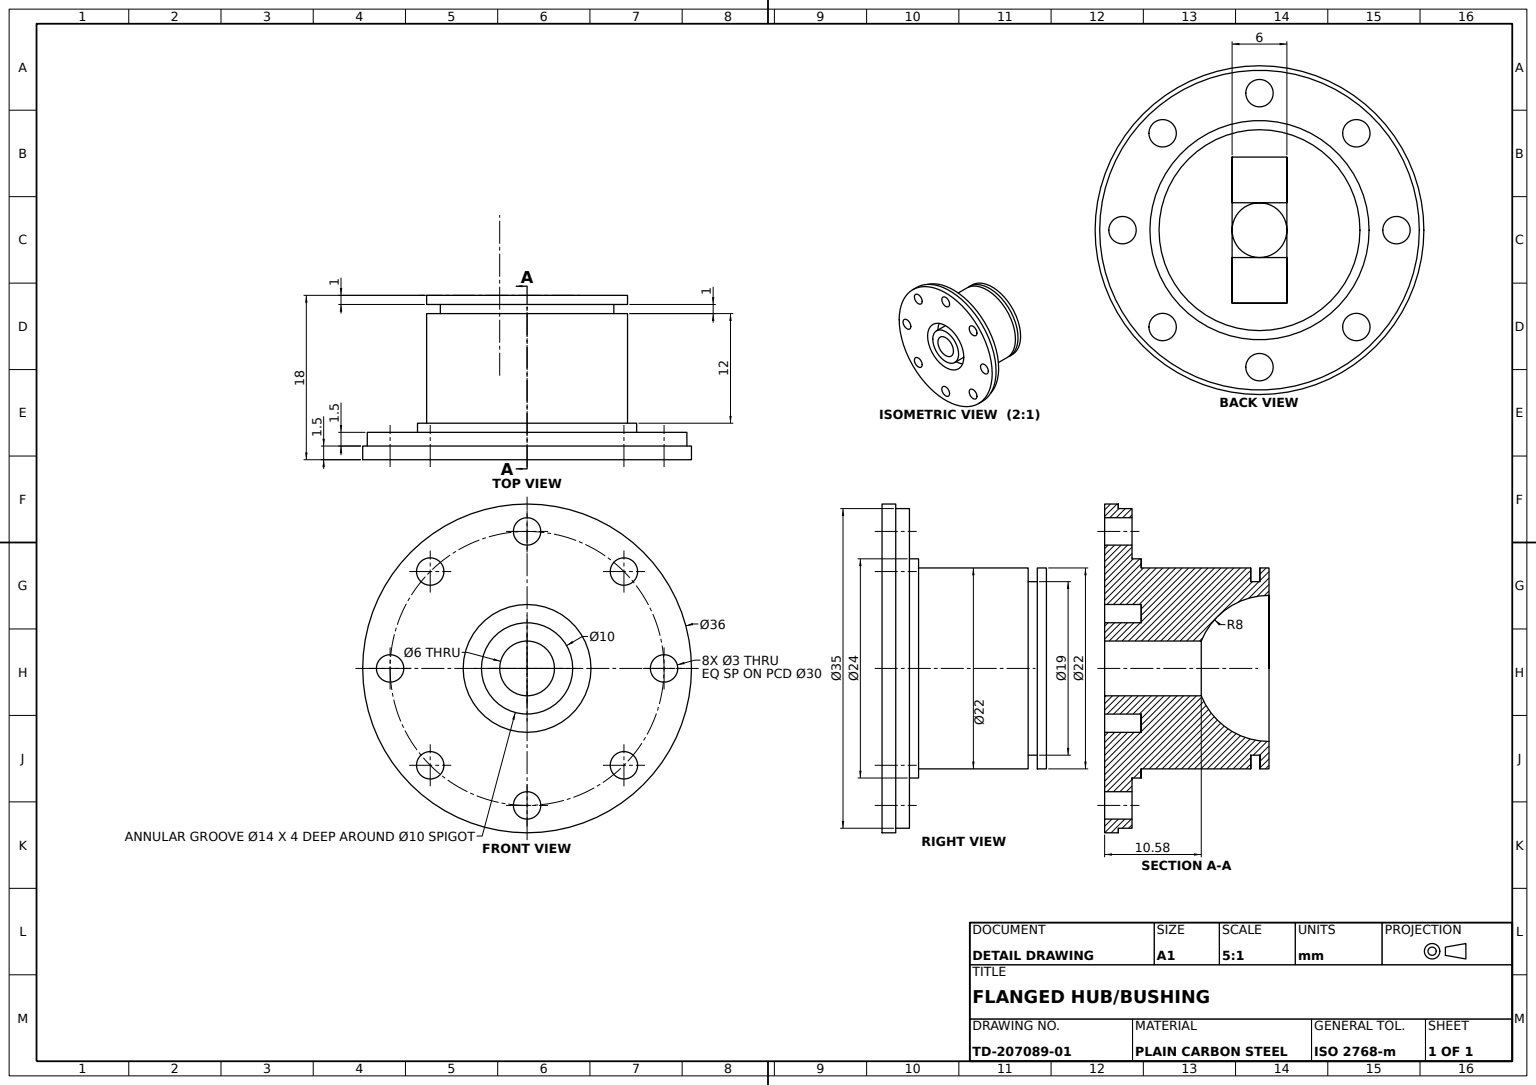
SolidWorks part; units mm, degrees
material "Plain Carbon Steel"
ref_plane "Front Plane" through (0, 0, 0) normal (0, 0, 1) x (1, 0, 0)
ref_plane "Top Plane" through (0, 0, 0) normal (0, 1, 0) x (1, 0, 0)
ref_plane "Right Plane" through (0, 0, 0) normal (1, 0, 0) x (0, 0, -1)
sketch "Base Lip Sketch Ø22" plane through (0, 0, 0) normal (0, 1, 0) x (1, 0, 0)
  circle A0 centre (0, 0) radius 11
  dimension "D1" = 22
extrude "Base Lip Ø22" add sketch "Base Lip Sketch Ø22" along normal blind 1
sketch "Groove Sketch Ø19" plane through (0, 1, 0) normal (0, 1, 0) x (1, 0, 0)
  circle A0 centre (0, 0) radius 9.5
  dimension "D1" = 19
extrude "Groove Neck Ø19" add sketch "Groove Sketch Ø19" along normal blind 1
sketch "Shank Sketch Ø22" plane through (0, 2, 0) normal (0, 1, 0) x (1, 0, 0)
  circle A0 centre (0, 0) radius 11
  dimension "D1" = 22
extrude "Shank Ø22" add sketch "Shank Sketch Ø22" along normal blind 12
sketch "Collar Sketch Ø24" plane through (0, 14, 0) normal (0, 1, 0) x (1, 0, 0)
  circle A0 centre (0, 0) radius 12
  dimension "D1" = 24
extrude "Collar Ø24" add sketch "Collar Sketch Ø24" along normal blind 1
sketch "Flange Lower Sketch Ø35" plane through (0, 15, 0) normal (0, 1, 0) x (1, 0, 0)
  circle A0 centre (0, 0) radius 17.5
  dimension "D1" = 35
extrude "Flange Lower Step Ø35" add sketch "Flange Lower Sketch Ø35" along normal blind 1.5
sketch "Flange Sketch Ø36" plane through (0, 16.5, 0) normal (0, 1, 0) x (1, 0, 0)
  circle A0 centre (0, 0) radius 18
  dimension "D1" = 36
extrude "Flange Ø36" add sketch "Flange Sketch Ø36" along normal blind 1.5
ref_plane "Window Cut Plane" through (0, 0, 0) normal (0, 0, 1) x (1, 0, 0)
sketch "Side Window Sketch" plane through (0, 0, 0) normal (0, 0, 1) x (1, 0, 0)
  line L0 (-8, 0) -> (8, 0)
  line L1 (-11, 0) -> (11, 0) construction
  line L2 (-3, 7.42) -> (3, 7.42)
  line L3 (18, 18) -> (-18, 18) construction
  arc A0 (-8, 0) -> (-3, 7.42) centre (0, 0.0038) cw
  arc A1 (3, 7.42) -> (8, 0) centre (0, 0.0038) cw
  point P6 (0, 0)
  point P9 (0, 7.42)
  dimension "D5" = 8
  dimension "D6" = 8
  dimension "D1" = 16
  dimension "D2" = 6
  dimension "D3" = 3
  dimension "D4" = 10.58
extrude "Side Window Cut" cut sketch "Side Window Sketch" against normal mid plane 6
sketch "Bolt Holes Sketch 8xØ3" plane through (0, 18, 0) normal (0, 1, 0) x (1, 0, 0)
  circle A1 centre (0, 15) radius 1.5
  circle A2 centre (10.6066, 10.6066) radius 1.5
  circle A3 centre (15, 0) radius 1.5
  circle A4 centre (10.6066, -10.6066) radius 1.5
  circle A5 centre (0, -15) radius 1.5
  circle A6 centre (-10.6066, -10.6066) radius 1.5
  circle A7 centre (-15, 0) radius 1.5
  circle A8 centre (-10.6066, 10.6066) radius 1.5
  dimension "D1" = 10.6066
  dimension "D2" = 3
  dimension "D4" = 15
  dimension "D5" = 10.6066
  dimension "D7" = 10.6066
  dimension "D3" = 8
extrude "Bolt Holes 8xØ3" cut sketch "Bolt Holes Sketch 8xØ3" against normal blind 6
sketch "Recess Sketch Ø14" plane through (0, 18, 0) normal (0, 1, 0) x (1, 0, 0)
  circle A0 centre (0, 0) radius 7
  dimension "D1" = 14
extrude "Recess Ø14" cut sketch "Recess Sketch Ø14" against normal blind 4
sketch "Inner Spigot Sketch Ø10" plane through (0, 18, 0) normal (0, 1, 0) x (1, 0, 0)
  circle A0 centre (0, 0) radius 5
  dimension "D1" = 10
extrude "Inner Spigot Ø10" add sketch "Inner Spigot Sketch Ø10" against normal blind 4
sketch "Bore Sketch Ø6" plane through (0, 18, 0) normal (0, 1, 0) x (1, 0, 0)
  circle A0 centre (0, 0) radius 3
  dimension "D1" = 6
extrude "Through Bore Ø6" cut sketch "Bore Sketch Ø6" against normal blind 10.58
